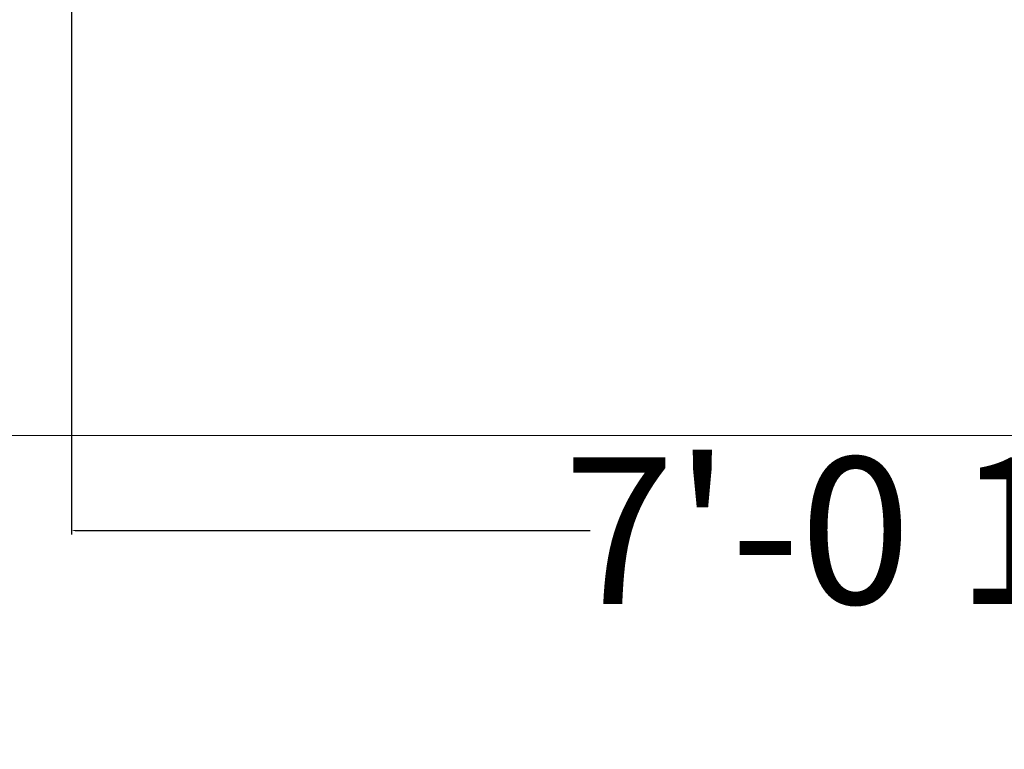
# Model space of a CAD drawing. Units: inches. Extents: x 1319 to 2030, y 219 to 1069.
# Tile 3 of 28: x 1417 to 1464, y 322 to 357. Entities that reach past the tile are written whole.
import ezdxf

# ---------------------------------------------------------------- set-up
doc = ezdxf.new("R2010")
doc.units = ezdxf.units.IN
doc.header["$MEASUREMENT"] = 0
doc.layers.add('A-ANNO-DIMS', color=2, linetype='Continuous', lineweight=18)
doc.layers.add('A-FLOR', color=8, linetype='Continuous', lineweight=18)
doc.styles.get("Standard").update_dxf_attribs({"font": 'arial.ttf'})
doc.dimstyles.get("Standard").update_dxf_attribs({"dimtxt": 7, "dimasz": 0.18, "dimexe": 0.18, "dimexo": 0.0625, "dimgap": 0.09, "dimtad": 0, "dimtih": 1, "dimtoh": 1, "dimzin": 0, "dimdsep": 46, "dimlunit": 3, "dimtxsty": 'Standard', "dimcen": 0.09, "dimadec": 0, "dimazin": 0, "dimtfac": 1, "dimtofl": 0, "dimtmove": 0, "dimatfit": 3, "dimfxl": 1, "dimtolj": 1, "dimtzin": 0, "dimarcsym": 0})

# ---------------------------------------------------------------- blocks, each defined once
blk = doc.blocks.new('*D57')
at = {"layer": 'A-ANNO-DIMS', "color": 0, "lineweight": -2, "transparency": 16777216}
for p, q in [((1419.914, 358.675), (1419.914, 332.688)), ((1504.443, 358.675), (1504.443, 332.688)), ((1420.094, 332.868), (1444.658, 332.868)), ((1504.263, 332.868), (1479.699, 332.868))]:
    blk.add_line(p, q, dxfattribs=at)
at = {"layer": 'A-ANNO-DIMS', "color": 0, "transparency": 16777216}
for points in [[(1420.094, 332.898), (1420.094, 332.838), (1419.914, 332.868)], [(1504.263, 332.898), (1504.263, 332.838), (1504.443, 332.868)]]:
    blk.add_solid(points, dxfattribs=at)
at = {"layer": 'Defpoints', "color": 0, "transparency": 16777216}
for p in [(1419.914, 358.738), (1504.443, 358.738), (1504.443, 332.868)]:
    blk.add_point(p, dxfattribs=at)
at = {"layer": 'A-ANNO-DIMS', "color": 0, "transparency": 16777216, "insert": (1462.179, 332.868), "char_height": 7, "attachment_point": 5}
blk.add_mtext('\\A1;7\'-0 1/2"', dxfattribs=at)

msp = doc.modelspace()

# ---------------------------------------------------------------- linework, layer by layer
at = {"layer": 'A-FLOR'}
msp.add_line((1394.092, 337.406), (1817.431, 337.406), dxfattribs=at)

# ---------------------------------------------------------------- dimensions: what is measured, and where the dimension line sits
at = {"layer": 'A-ANNO-DIMS'}
dim = msp.add_linear_dim(base=(1504.443, 332.868), p1=(1419.914, 358.738), p2=(1504.443, 358.738), dimstyle='Standard', override={"dimdec": 1, "dimlfac": 1, "dimrnd": 0, "dimzin": 1, "dimdsep": 46, "dimlunit": 4, "dimfrac": 2}, dxfattribs=at)
dim.commit()
dim.dimension.update_dxf_attribs({"geometry": '*D57', "text_midpoint": (1462.179, 332.868)})

doc.saveas('drawing.dxf')
